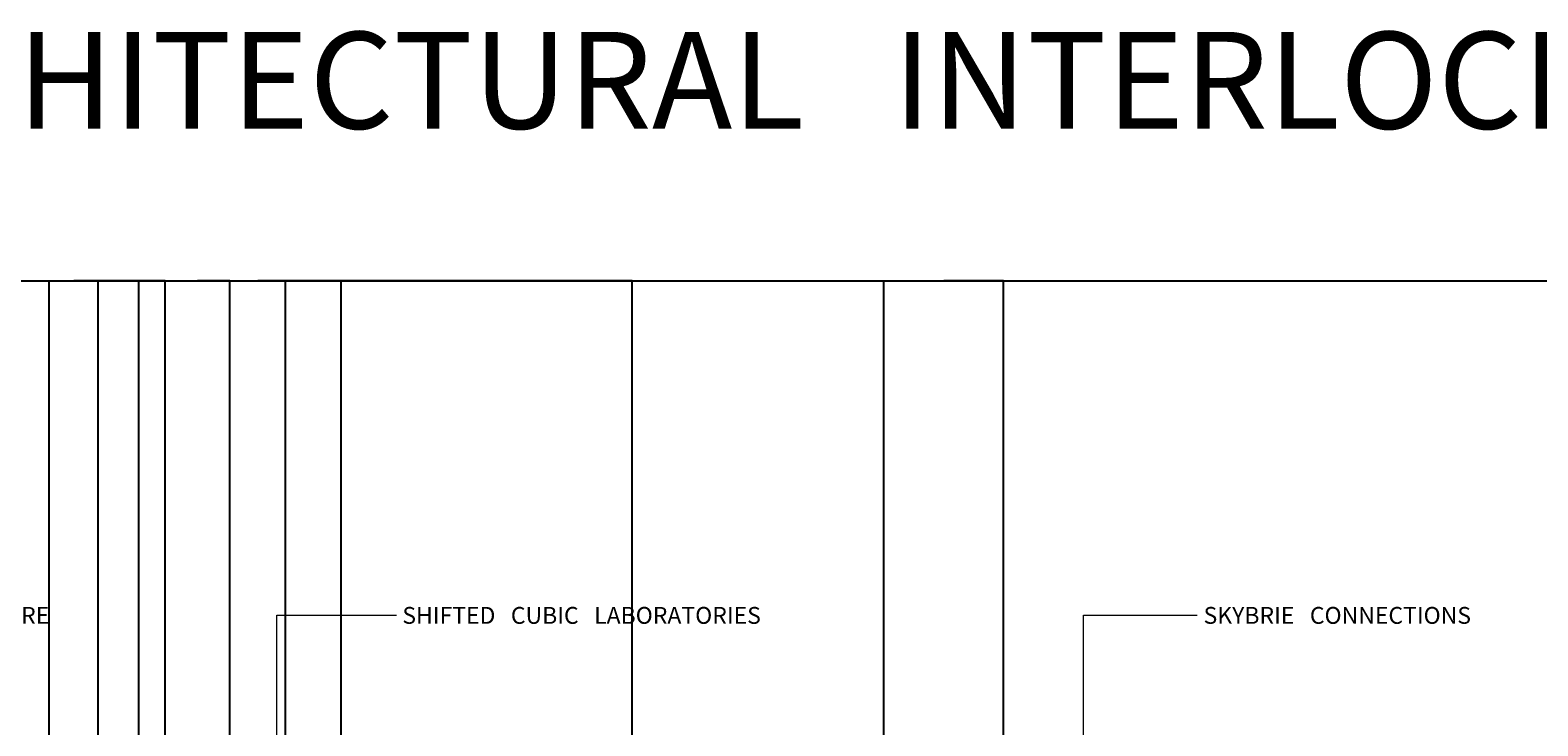
# Model space of a CAD drawing. Units: inches. Extents: x -32109 to 33221, y -19197 to 7608.
# Tile 13 of 25: x -11787 to -741, y 2510 to 7608. Entities that reach past the tile are written whole.
import ezdxf

# ---------------------------------------------------------------- set-up
doc = ezdxf.new("R2010")
doc.units = ezdxf.units.IN
doc.header["$MEASUREMENT"] = 0
for name, color, linetype, lineweight in [('A-ANNO-DIMS', 2, 'Continuous', 18), ('A-ANNO-NOTE', 2, 'Continuous', 18), ('A-ANNO-TEXT', 7, 'Continuous', 25)]:
    doc.layers.add(name, color=color, linetype=linetype, lineweight=lineweight)
doc.styles.get("Standard").update_dxf_attribs({"font": 'arial.ttf'})
doc.dimstyles.get("Standard").update_dxf_attribs({"dimtxt": 0.18, "dimasz": 0.18, "dimexe": 0.18, "dimexo": 0.0625, "dimgap": 0.09, "dimtad": 0, "dimtih": 1, "dimtoh": 1, "dimdec": 4, "dimzin": 0, "dimdsep": 46, "dimtxsty": 'Standard', "dimcen": 0.09, "dimadec": 0, "dimazin": 0, "dimtfac": 1, "dimtdec": 4, "dimtofl": 0, "dimtmove": 0, "dimatfit": 3, "dimfxl": 1, "dimtolj": 1, "dimtzin": 0, "dimarcsym": 0})

# ---------------------------------------------------------------- blocks, each defined once
blk = doc.blocks.new('*D10')
at = {"layer": 'A-ANNO-DIMS', "color": 0, "lineweight": -2, "transparency": 16777216}
for p, q in [((-18512.646816, -110.179138), (-18512.646816, 5772.015489000001)), ((-18512.466816, 5771.835489), (-202.0927503703958, 5771.835489)), ((18109.136745, 5771.835489), (-201.2373206296045, 5771.835489)), ((18109.316745, -101.537382), (18109.316745, 5772.015489000001))]:
    blk.add_line(p, q, dxfattribs=at)
at = {"layer": 'A-ANNO-DIMS', "color": 0, "transparency": 16777216}
for points in [[(-18512.466816, 5771.865488999999), (-18512.466816, 5771.805489000001), (-18512.646816, 5771.835489)], [(18109.136745, 5771.865488999999), (18109.136745, 5771.805489000001), (18109.316745, 5771.835489)]]:
    blk.add_solid(points, dxfattribs=at)
at = {"layer": 'Defpoints', "color": 0, "transparency": 16777216}
for p in [(18109.316745, 5771.835489), (-18512.646816, -110.241638), (18109.316745, -101.599882)]:
    blk.add_point(p, dxfattribs=at)
at = {"layer": 'A-ANNO-DIMS', "color": 0, "transparency": 16777216, "insert": (-201.6650355000002, 5771.835489), "char_height": 0.18, "attachment_point": 5}
blk.add_mtext('\\A1;36622', dxfattribs=at)
blk = doc.blocks.new('*D20')
at = {"layer": 'A-ANNO-DIMS', "color": 0, "lineweight": -2, "transparency": 16777216}
for p, q in [((-5532.1011, -1149.167073), (-5532.1011, 5772.015489)), ((-5531.921099999999, 5771.835489), (-5094.412020594814, 5771.835489)), ((-4656.325124, 5771.835489), (-5093.834203405184, 5771.835489)), ((-4656.145124, -1149.167073), (-4656.145124, 5772.015489))]:
    blk.add_line(p, q, dxfattribs=at)
at = {"layer": 'A-ANNO-DIMS', "color": 0, "transparency": 16777216}
for points in [[(-5531.921099999999, 5771.865488999999), (-5531.921099999999, 5771.805489000001), (-5532.1011, 5771.835489)], [(-4656.325124, 5771.865488999999), (-4656.325124, 5771.805489000001), (-4656.145124, 5771.835489)]]:
    blk.add_solid(points, dxfattribs=at)
at = {"layer": 'Defpoints', "color": 0, "transparency": 16777216}
for p in [(-4656.145124, 5771.835489), (-5532.1011, -1149.229573), (-4656.145124, -1149.229573)]:
    blk.add_point(p, dxfattribs=at)
at = {"layer": 'A-ANNO-DIMS', "color": 0, "transparency": 16777216, "insert": (-5094.123112, 5771.835489), "char_height": 0.18, "attachment_point": 5}
blk.add_mtext('\\A1;876', dxfattribs=at)
blk = doc.blocks.new('*D44')
at = {"layer": 'A-ANNO-DIMS', "color": 0, "lineweight": -2, "transparency": 16777216}
for p, q in [((-12501.358719, 764.249093), (-12501.358719, 5772.015489000001)), ((-12501.178719, 5771.835489), (-9938.977615976126, 5771.835489)), ((-7376.057618000001, 5771.835489), (-9938.258721023878, 5771.835489)), ((-7375.877618000001, 764.249093), (-7375.877618000001, 5772.015489000001))]:
    blk.add_line(p, q, dxfattribs=at)
at = {"layer": 'A-ANNO-DIMS', "color": 0, "transparency": 16777216}
for points in [[(-12501.178719, 5771.865488999999), (-12501.178719, 5771.805489000001), (-12501.358719, 5771.835489)], [(-7376.057618000001, 5771.865488999999), (-7376.057618000001, 5771.805489000001), (-7375.877618000001, 5771.835489)]]:
    blk.add_solid(points, dxfattribs=at)
at = {"layer": 'Defpoints', "color": 0, "transparency": 16777216}
for p in [(-7375.877618000001, 5771.835489), (-12501.358719, 764.186593), (-7375.877618000001, 764.186593)]:
    blk.add_point(p, dxfattribs=at)
at = {"layer": 'A-ANNO-DIMS', "color": 0, "transparency": 16777216, "insert": (-9938.618168500001, 5771.835489), "char_height": 0.18, "attachment_point": 5}
blk.add_mtext('\\A1;5125', dxfattribs=at)
blk = doc.blocks.new('*D45')
at = {"layer": 'A-ANNO-DIMS', "color": 0, "lineweight": -2, "transparency": 16777216}
for p, q in [((-11898.560127, 598.986194), (-11898.560127, 5772.015489000001)), ((-11898.380127, 5771.835489), (-11444.88544065006, 5771.835489)), ((-10990.638094, 5771.835489), (-11444.13278034993, 5771.835489)), ((-10990.458094, 598.060066), (-10990.458094, 5772.015489000001))]:
    blk.add_line(p, q, dxfattribs=at)
at = {"layer": 'A-ANNO-DIMS', "color": 0, "transparency": 16777216}
for points in [[(-11898.380127, 5771.865488999999), (-11898.380127, 5771.805489000001), (-11898.560127, 5771.835489)], [(-10990.638094, 5771.865488999999), (-10990.638094, 5771.805489000001), (-10990.458094, 5771.835489)]]:
    blk.add_solid(points, dxfattribs=at)
at = {"layer": 'Defpoints', "color": 0, "transparency": 16777216}
for p in [(-10990.458094, 5771.835489), (-11898.560127, 598.923694), (-10990.458094, 597.997566)]:
    blk.add_point(p, dxfattribs=at)
at = {"layer": 'A-ANNO-DIMS', "color": 0, "transparency": 16777216, "insert": (-11444.5091105, 5771.835489), "char_height": 0.18, "attachment_point": 5}
blk.add_mtext('\\A1;908.1', dxfattribs=at)
blk = doc.blocks.new('*D48')
at = {"layer": 'A-ANNO-DIMS', "color": 0, "lineweight": -2, "transparency": 16777216}
for p, q in [((-11646.505496, -179.616281), (-11646.505496, 5772.015489000001)), ((-11646.325496, 5771.835489), (-11468.09538433765, 5771.835489)), ((-11288.936787, 5771.835489), (-11467.16689866234, 5771.835489)), ((-11288.756787, -179.616281), (-11288.756787, 5772.015489000001))]:
    blk.add_line(p, q, dxfattribs=at)
at = {"layer": 'A-ANNO-DIMS', "color": 0, "transparency": 16777216}
for points in [[(-11646.325496, 5771.865488999999), (-11646.325496, 5771.805489000001), (-11646.505496, 5771.835489)], [(-11288.936787, 5771.865488999999), (-11288.936787, 5771.805489000001), (-11288.756787, 5771.835489)]]:
    blk.add_solid(points, dxfattribs=at)
at = {"layer": 'Defpoints', "color": 0, "transparency": 16777216}
for p in [(-11288.756787, 5771.835489), (-11646.505496, -179.678781), (-11288.756787, -179.678781)]:
    blk.add_point(p, dxfattribs=at)
at = {"layer": 'A-ANNO-DIMS', "color": 0, "transparency": 16777216, "insert": (-11467.6311415, 5771.835489), "char_height": 0.18, "attachment_point": 5}
blk.add_mtext('\\A1;357.75', dxfattribs=at)
blk = doc.blocks.new('*D49')
at = {"layer": 'A-ANNO-DIMS', "color": 0, "lineweight": -2, "transparency": 16777216}
for p, q in [((-11288.756787, -179.616281), (-11288.756787, 5772.015489000001)), ((-11288.576787, 5771.835489), (-11043.72206223192, 5771.835489)), ((-10798.072317, 5771.835489), (-11042.92704176807, 5771.835489)), ((-10797.892317, -179.616281), (-10797.892317, 5772.015489000001))]:
    blk.add_line(p, q, dxfattribs=at)
at = {"layer": 'A-ANNO-DIMS', "color": 0, "transparency": 16777216}
for points in [[(-11288.576787, 5771.865488999999), (-11288.576787, 5771.805489000001), (-11288.756787, 5771.835489)], [(-10798.072317, 5771.865488999999), (-10798.072317, 5771.805489000001), (-10797.892317, 5771.835489)]]:
    blk.add_solid(points, dxfattribs=at)
at = {"layer": 'Defpoints', "color": 0, "transparency": 16777216}
for p in [(-10797.892317, 5771.835489), (-11288.756787, -179.678781), (-10797.892317, -179.678781)]:
    blk.add_point(p, dxfattribs=at)
at = {"layer": 'A-ANNO-DIMS', "color": 0, "transparency": 16777216, "insert": (-11043.324552, 5771.835489), "char_height": 0.18, "attachment_point": 5}
blk.add_mtext('\\A1;490.9', dxfattribs=at)
blk = doc.blocks.new('*D50')
at = {"layer": 'A-ANNO-DIMS', "color": 0, "lineweight": -2, "transparency": 16777216}
for p, q in [((-10797.892317, -179.616281), (-10797.892317, 5772.015489000001)), ((-10797.712317, 5771.835489), (-10561.17616518417, 5771.835489)), ((-10323.847203, 5771.835489), (-10560.38335481582, 5771.835489)), ((-10323.667203, -179.616281), (-10323.667203, 5772.015489000001))]:
    blk.add_line(p, q, dxfattribs=at)
at = {"layer": 'A-ANNO-DIMS', "color": 0, "transparency": 16777216}
for points in [[(-10797.712317, 5771.865488999999), (-10797.712317, 5771.805489000001), (-10797.892317, 5771.835489)], [(-10323.847203, 5771.865488999999), (-10323.847203, 5771.805489000001), (-10323.667203, 5771.835489)]]:
    blk.add_solid(points, dxfattribs=at)
at = {"layer": 'Defpoints', "color": 0, "transparency": 16777216}
for p in [(-10323.667203, 5771.835489), (-10797.892317, -179.678781), (-10323.667203, -179.678781)]:
    blk.add_point(p, dxfattribs=at)
at = {"layer": 'A-ANNO-DIMS', "color": 0, "transparency": 16777216, "insert": (-10560.77976, 5771.835489), "char_height": 0.18, "attachment_point": 5}
blk.add_mtext('\\A1;474.2', dxfattribs=at)
blk = doc.blocks.new('*D51')
at = {"layer": 'A-ANNO-DIMS', "color": 0, "lineweight": -2, "transparency": 16777216}
for p, q in [((-10323.667203, -179.616281), (-10323.667203, 5772.015489000001)), ((-10323.487203, 5771.835489), (-10120.2309580573, 5771.835489)), ((-9916.180061000003, 5771.835489), (-10119.4363059427, 5771.835489)), ((-9916.000061, -179.616281), (-9916.000061, 5772.015489000001))]:
    blk.add_line(p, q, dxfattribs=at)
at = {"layer": 'A-ANNO-DIMS', "color": 0, "transparency": 16777216}
for points in [[(-10323.487203, 5771.865488999999), (-10323.487203, 5771.805489000001), (-10323.667203, 5771.835489)], [(-9916.180061000003, 5771.865488999999), (-9916.180061000003, 5771.805489000001), (-9916.000061, 5771.835489)]]:
    blk.add_solid(points, dxfattribs=at)
at = {"layer": 'Defpoints', "color": 0, "transparency": 16777216}
for p in [(-9916.000061, 5771.835489), (-10323.667203, -179.678781), (-9916.000061, -179.678781)]:
    blk.add_point(p, dxfattribs=at)
at = {"layer": 'A-ANNO-DIMS', "color": 0, "transparency": 16777216, "insert": (-10119.833632, 5771.835489), "char_height": 0.18, "attachment_point": 5}
blk.add_mtext('\\A1;407.7', dxfattribs=at)
blk = doc.blocks.new('*D52')
at = {"layer": 'A-ANNO-DIMS', "color": 0, "lineweight": -2, "transparency": 16777216}
for p, q in [((-9916.000061, -179.616281), (-9916.000061, 5772.015489000001)), ((-9915.820061, 5771.835489), (-9712.563908057302, 5771.835489)), ((-9508.513103000001, 5771.835489), (-9711.769255942705, 5771.835489)), ((-9508.333103, -179.616281), (-9508.333103, 5772.015489000001))]:
    blk.add_line(p, q, dxfattribs=at)
at = {"layer": 'A-ANNO-DIMS', "color": 0, "transparency": 16777216}
for points in [[(-9915.820061, 5771.865488999999), (-9915.820061, 5771.805489000001), (-9916.000061, 5771.835489)], [(-9508.513103000001, 5771.865488999999), (-9508.513103000001, 5771.805489000001), (-9508.333103, 5771.835489)]]:
    blk.add_solid(points, dxfattribs=at)
at = {"layer": 'Defpoints', "color": 0, "transparency": 16777216}
for p in [(-9508.333103, 5771.835489), (-9916.000061, -179.678781), (-9508.333103, -179.678781)]:
    blk.add_point(p, dxfattribs=at)
at = {"layer": 'A-ANNO-DIMS', "color": 0, "transparency": 16777216, "insert": (-9712.166582000002, 5771.835489), "char_height": 0.18, "attachment_point": 5}
blk.add_mtext('\\A1;407.7', dxfattribs=at)

msp = doc.modelspace()

# ---------------------------------------------------------------- linework, layer by layer
at = {"layer": 'A-ANNO-NOTE'}
for p, q in [((-9978.983117329653, 1074.546111827018), (-9978.983117329653, 3321.835488633431)), ((-9978.983117329653, 3321.835488633431), (-9102.910564633203, 3321.835488633431)), ((-4070.255914539331, 1242.026295574848), (-4070.255914539331, 3321.835488633435)), ((-4070.255914539331, 3321.835488633435), (-3235.900959998951, 3321.835488633435))]:
    msp.add_line(p, q, dxfattribs=at)

# ---------------------------------------------------------------- texts
at = {"layer": 'A-ANNO-TEXT'}
for s, height, p in [('COMPREHENSIVE   ARCHITECTURAL   INTERLOCKING    CUBE   MEGA   CAMPUC   MASTER   PLAN ', 709.7949465747753, (-22238.10681632875, 6885.298304043546)), ('COLOSSAL   RESEARCH    CORE ', 123.5547426012344, (-14039.9432806184, 3257.545255676414)), ('SHIFTED   CUBIC   LABORATORIES', 123.5547426012344, (-9060.104397596559, 3257.545255676414)), ('SKYBRIE   CONNECTIONS', 123.5547426012344, (-3189.73168881028, 3257.545255676414))]:
    msp.add_text(s, height=height, dxfattribs=at).set_placement(p)

# ---------------------------------------------------------------- dimensions: what is measured, and where the dimension line sits
at = {"layer": 'A-ANNO-DIMS'}
for base, p1, p2, override, picture, middle in [((18109.316745, 5771.835489), (-18512.646816, -110.241638), (18109.316745, -101.599882), {"dimdec": 0, "dimlfac": 1, "dimrnd": 0, "dimzin": 0, "dimdsep": 46, "dimlunit": 2}, '*D10', (-201.6650355000002, 5771.835489)), ((-7375.877618000001, 5771.835489), (-12501.358719, 764.186593), (-7375.877618000001, 764.186593), {"dimdec": 0, "dimlfac": 1, "dimrnd": 0, "dimzin": 0, "dimdsep": 46, "dimlunit": 2}, '*D44', (-9938.618168500001, 5771.835489)), ((-10990.458094, 5771.835489), (-11898.560127, 598.923694), (-10990.458094, 597.997566), {"dimdec": 1, "dimlfac": 1, "dimrnd": 0, "dimzin": 0, "dimdsep": 46, "dimlunit": 2}, '*D45', (-11444.5091105, 5771.835489)), ((-11288.756787, 5771.835489), (-11646.505496, -179.678781), (-11288.756787, -179.678781), {"dimdec": 2, "dimlfac": 1, "dimrnd": 0, "dimzin": 0, "dimdsep": 46, "dimlunit": 2}, '*D48', (-11467.6311415, 5771.835489)), ((-10797.892317, 5771.835489), (-11288.756787, -179.678781), (-10797.892317, -179.678781), {"dimdec": 1, "dimlfac": 1, "dimrnd": 0, "dimzin": 0, "dimdsep": 46, "dimlunit": 2}, '*D49', (-11043.324552, 5771.835489)), ((-10323.667203, 5771.835489), (-10797.892317, -179.678781), (-10323.667203, -179.678781), {"dimdec": 1, "dimlfac": 1, "dimrnd": 0, "dimzin": 0, "dimdsep": 46, "dimlunit": 2}, '*D50', (-10560.77976, 5771.835489)), ((-9916.000061, 5771.835489), (-10323.667203, -179.678781), (-9916.000061, -179.678781), {"dimdec": 1, "dimlfac": 1, "dimrnd": 0, "dimzin": 0, "dimdsep": 46, "dimlunit": 2}, '*D51', (-10119.833632, 5771.835489)), ((-9508.333103, 5771.835489), (-9916.000061, -179.678781), (-9508.333103, -179.678781), {"dimdec": 1, "dimlfac": 1, "dimrnd": 0, "dimzin": 0, "dimdsep": 46, "dimlunit": 2}, '*D52', (-9712.166582000002, 5771.835489)), ((-4656.145124, 5771.835489), (-5532.1011, -1149.229573), (-4656.145124, -1149.229573), {"dimdec": 0, "dimlfac": 1, "dimrnd": 0, "dimzin": 0, "dimdsep": 46, "dimlunit": 2}, '*D20', (-5094.123112, 5771.835489))]:
    dim = msp.add_linear_dim(base=base, p1=p1, p2=p2, dimstyle='Standard', override=override, dxfattribs=at)
    dim.commit()
    dim.dimension.update_dxf_attribs({"geometry": picture, "text_midpoint": middle})

doc.saveas('drawing.dxf')
